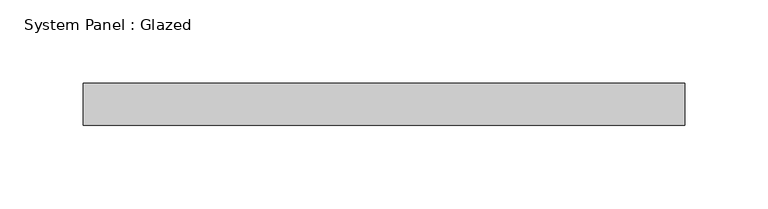
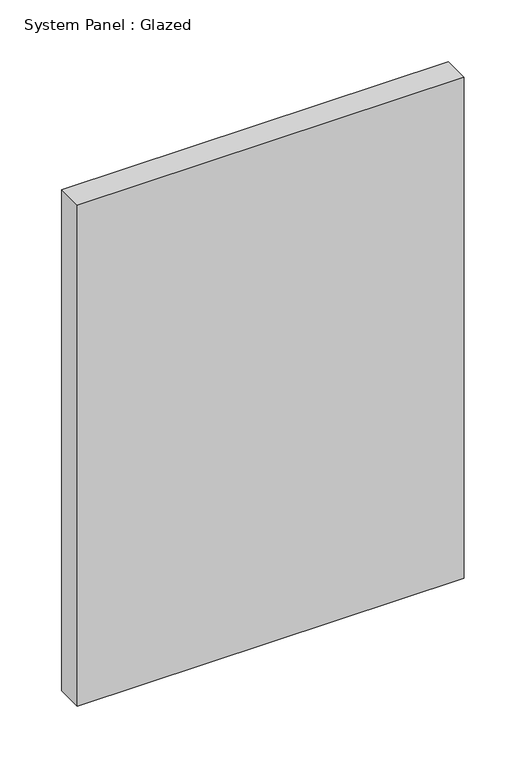
"""IFC4 building model written with IfcOpenShell, lengths in millimetres: plate geometry, System Panel : Glazed."""

from ifc_helpers import new_model, si_unit, origin, origin_with_axes, place, context, project, spatial, polyline, outline, extrude, source, transform, mapped, element, save


def system_panel_glazed_6c61ac18(model_context):
    return source(origin(), model_context, "Body", "SweptSolid", [
        extrude(outline(polyline([(180.975, 19.05), (-180.975, 19.05), (-180.975, 44.45), (180.975, 44.45), (180.975, 19.05)])), origin_with_axes(), (0.0, 0.0, 1.0), 495.3),
    ])


if __name__ == "__main__":
    model = new_model("IFC4")
    model_context = context("Model", 3, world=origin())
    ifc_project = project(units=[si_unit("LENGTHUNIT", "METRE", prefix="MILLI")], contexts=[model_context])
    site = spatial("IfcSite", under=ifc_project)
    building = spatial("IfcBuilding", under=site)
    placement = place(None, origin())
    system_panel_glazed_shape = system_panel_glazed_6c61ac18(model_context)
    element("IfcPlate", 1, ObjectType="System Panel : Glazed", at=placement, inside=building, context=model_context, shape_type="MappedRepresentation", body=[
        mapped(system_panel_glazed_shape, transform((0.0, 0.0, 0.0), x_axis=(1.0, 0.0, 0.0), y_axis=(0.0, 1.0, 0.0), z_axis=(0.0, 0.0, 1.0))),
    ])
    save(model, "model.ifc")

# Revit data of these elements
# Type "System Panel : Glazed"
#   Construction Type Id = "GSP4R"
#   Analytic Construction = "1/8 in Pilkington single glazing"
#   Visual Light Transmittance = 0.9
#   Solar Heat Gain Coefficient = 0.86
#   Heat Transfer Coefficient (U) = 1.18115 BTU/(h·ft²·°F)
#   Define Thermal Properties by = 1
# Element 1 (IfcPlate, "System Panel : Glazed")
#   Materials on its faces: "Glass"
# Materials
#   "Glass": class "Glass", colour RGB 0 128 192, transparency 0.75, Description = "Soda Lime Glass", Cost = 0
